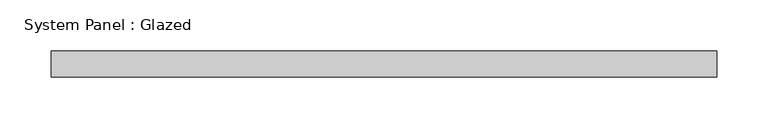
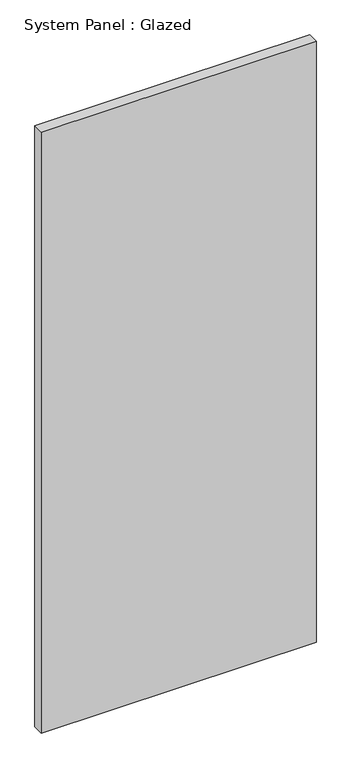
"""IFC4 building model written with IfcOpenShell, lengths in millimetres: plate geometry, System Panel : Glazed."""

from ifc_helpers import new_model, si_unit, origin, origin_with_axes, place, context, project, spatial, polyline, outline, extrude, source, transform, mapped, element, save


def system_panel_glazed_98683e45(model_context):
    return source(origin(), model_context, "Body", "SweptSolid", [
        extrude(outline(polyline([(323.85, 19.05), (-323.85, 19.05), (-323.85, 44.45), (323.85, 44.45), (323.85, 19.05)])), origin_with_axes(), (0.0, 0.0, 1.0), 1496.9353791),
    ])


if __name__ == "__main__":
    model = new_model("IFC4")
    model_context = context("Model", 3, world=origin())
    ifc_project = project(units=[si_unit("LENGTHUNIT", "METRE", prefix="MILLI")], contexts=[model_context])
    site = spatial("IfcSite", under=ifc_project)
    building = spatial("IfcBuilding", under=site)
    placement = place(None, origin())
    system_panel_glazed_shape = system_panel_glazed_98683e45(model_context)
    element("IfcPlate", 1, ObjectType="System Panel : Glazed", at=placement, inside=building, context=model_context, shape_type="MappedRepresentation", body=[
        mapped(system_panel_glazed_shape, transform((0.0, 0.0, 0.0), x_axis=(1.0, 0.0, 0.0), y_axis=(0.0, 1.0, 0.0), z_axis=(0.0, 0.0, 1.0))),
    ])
    save(model, "model.ifc")

# Revit data of these elements
# Type "System Panel : Glazed"
#   Construction Type Id = "GSP4R"
#   Analytic Construction = "1/8 in Pilkington single glazing"
#   Visual Light Transmittance = 0.9
#   Solar Heat Gain Coefficient = 0.86
#   Heat Transfer Coefficient (U) = 1.18115 BTU/(h·ft²·°F)
#   Define Thermal Properties by = 1
# Element 1 (IfcPlate, "System Panel : Glazed")
#   Materials on its faces: "Glass"
# Materials
#   "Glass": class "Glass", colour RGB 0 128 192, transparency 0.75, Description = "Soda Lime Glass", Cost = 0
